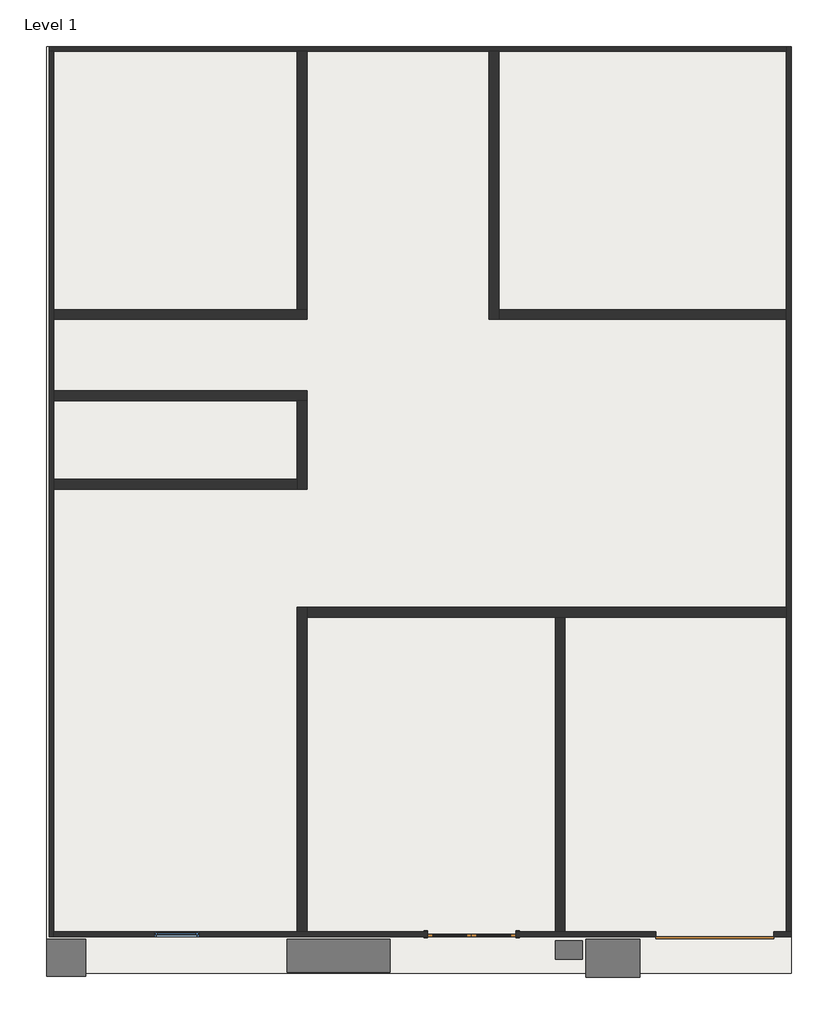
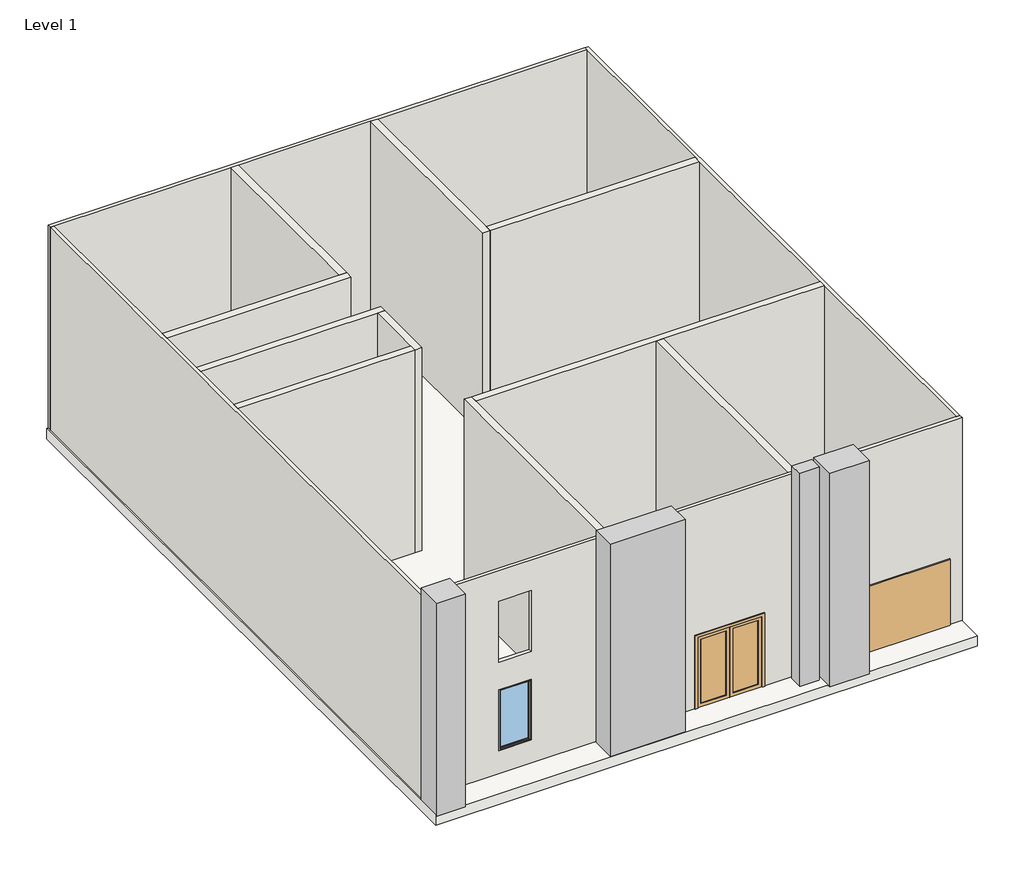
# One storey: 14 walls, 4 proxies, 2 doors, 1 slab, 1 window.
"""IFC4 building model written with IfcOpenShell, lengths in millimetres."""

from ifc_helpers import new_model, si_unit, frame, origin, origin_with_axes, place, context, project, spatial, polyline, outline, extrude, faceted_brep, transform, mapped, element, save
from components import generic_models_4_generic_models_4_105e3c89, generic_models_6_generic_models_6_789752cf, generic_models_7_generic_models_7_5b8c9dda, generic_models_8_generic_models_8_60fedc48, door_8f551b21, door_8b017a1a, window_8ce0b82f

model = new_model("IFC4")

# Units and contexts
model_context = context("Model", 3, world=origin())
ifc_project = project(units=[si_unit("LENGTHUNIT", "METRE", prefix="MILLI")], contexts=[model_context])

# Site, building, storey
site = spatial("IfcSite", under=ifc_project)
building = spatial("IfcBuilding", under=site)
storey = spatial("IfcBuildingStorey", under=building, Name="Level 1", Elevation=0.0)

# Proxies
placement = place(None, origin())
generic_models_4_generic_models_4_shape = generic_models_4_generic_models_4_105e3c89(model_context)
element("IfcBuildingElementProxy", 1, Name="Generic Models 4 : Generic Models 4", ObjectType="Generic Models 4 : Generic Models 4", at=placement, inside=storey, context=model_context, shape_type="MappedRepresentation", body=[
    mapped(generic_models_4_generic_models_4_shape, transform((0.0, 0.0, 0.0), x_axis=(1.0, 0.0, 0.0), y_axis=(0.0, 1.0, 0.0), z_axis=(0.0, 0.0, 1.0))),
])
generic_models_6_generic_models_6_shape = generic_models_6_generic_models_6_789752cf(model_context)
element("IfcBuildingElementProxy", 2, Name="Generic Models 6 : Generic Models 6", ObjectType="Generic Models 6 : Generic Models 6", at=placement, inside=storey, context=model_context, shape_type="MappedRepresentation", body=[
    mapped(generic_models_6_generic_models_6_shape, transform((0.0, 0.0, 0.0), x_axis=(1.0, 0.0, 0.0), y_axis=(0.0, 1.0, 0.0), z_axis=(0.0, 0.0, 1.0))),
])
generic_models_7_generic_models_7_shape = generic_models_7_generic_models_7_5b8c9dda(model_context)
element("IfcBuildingElementProxy", 3, Name="Generic Models 7 : Generic Models 7", ObjectType="Generic Models 7 : Generic Models 7", at=placement, inside=storey, context=model_context, shape_type="MappedRepresentation", body=[
    mapped(generic_models_7_generic_models_7_shape, transform((0.0, 0.0, 0.0), x_axis=(1.0, 0.0, 0.0), y_axis=(0.0, 1.0, 0.0), z_axis=(0.0, 0.0, 1.0))),
])
generic_models_8_generic_models_8_shape = generic_models_8_generic_models_8_60fedc48(model_context)
element("IfcBuildingElementProxy", 4, Name="Generic Models 8 : Generic Models 8", ObjectType="Generic Models 8 : Generic Models 8", at=placement, inside=storey, context=model_context, shape_type="MappedRepresentation", body=[
    mapped(generic_models_8_generic_models_8_shape, transform((0.0, 0.0, 0.0), x_axis=(1.0, 0.0, 0.0), y_axis=(0.0, 1.0, 0.0), z_axis=(0.0, 0.0, 1.0))),
])

# Doors
door_shape = door_8f551b21(model_context)
element("IfcDoor", 5, ObjectType="Door-Double-Glass : 72\" x 84\"", at=placement, inside=storey, context=model_context, shape_type="MappedRepresentation", body=[
    mapped(door_shape, transform((-1674.8069895, -8388.8167799, 0.0), x_axis=(-1.0, 0.0, 0.0), y_axis=(0.0, -1.0, 0.0), z_axis=(0.0, 0.0, 1.0))),
])
door_2_shape = door_8b017a1a(model_context)
element("IfcDoor", 6, ObjectType="Door-Overhead-Sectional : 8' x 6'-6\"", at=placement, inside=storey, context=model_context, shape_type="MappedRepresentation", body=[
    mapped(door_2_shape, transform((3354.3930105, -8391.1980299, 0.0), x_axis=(-1.0, 0.0, 0.0), y_axis=(0.0, -1.0, 0.0), z_axis=(0.0, 0.0, 1.0))),
])

# Slab
element("IfcSlab", 7, ObjectType="Generic - 12\"", at=placement, inside=storey, context=model_context, shape_type="SweptSolid", body=[
    extrude(outline(polyline([(4929.1930105, 9947.6019701), (4929.1930105, -9200.130387), (-10463.2069895, -9200.130387), (-10463.2069895, 9947.6019701), (4929.1930105, 9947.6019701)])), frame((0.0, 0.0, -304.8), z_axis=(0.0, 0.0, 1.0), x_axis=(1.0, 0.0, 0.0)), (0.0, 0.0, 1.0), 304.8),
])

# Walls
element("IfcWall", 8, ObjectType="Generic - 4\" Brick", at=placement, inside=storey, context=model_context, shape_type="Brep", body=[
    faceted_brep([(-10412.4069895, 9846.0019701, 0.0), (-10310.8069895, 9846.0019701, 0.0), (-5281.6069895, 9846.0019701, 0.0), (-5078.4069895, 9846.0019701, 0.0), (-1319.2069895, 9846.0019701, 0.0), (-1116.0069895, 9846.0019701, 0.0), (4827.5930105, 9846.0019701, 0.0), (4827.5930105, 9846.0019701, 6096.0), (-1116.0069895, 9846.0019701, 6096.0), (-1319.2069895, 9846.0019701, 6096.0), (-5078.4069895, 9846.0019701, 6096.0), (-5281.6069895, 9846.0019701, 6096.0), (-10310.8069895, 9846.0019701, 6096.0), (-10412.4069895, 9846.0019701, 6096.0), (-10412.4069895, 9947.6019701, 0.0), (-10412.4069895, 9947.6019701, 6096.0), (4827.5930105, 9947.6019701, 6096.0), (4827.5930105, 9947.6019701, 0.0)], [[[0, 1, 2, 3, 4, 5, 6, 7, 8, 9, 10, 11, 12, 13]], [[14, 15, 16, 17]], [[6, 5, 4, 3, 2, 1, 0, 14, 17]], [[0, 13, 15, 14]], [[7, 6, 17, 16]], [[13, 12, 11, 10, 9, 8, 7, 16, 15]]]),
])
element("IfcWall", 9, ObjectType="Generic - 4\" Brick", at=placement, inside=storey, context=model_context, shape_type="Brep", body=[
    faceted_brep([(-10310.8069895, -8441.9980299, 0.0), (-10310.8069895, -8340.3980299, 0.0), (-10310.8069895, 803.6019701, 0.0), (-10310.8069895, 1006.8019701, 0.0), (-10310.8069895, 2632.4019701, 0.0), (-10310.8069895, 2835.6019701, 0.0), (-10310.8069895, 4308.8019701, 0.0), (-10310.8069895, 4512.0019701, 0.0), (-10310.8069895, 9846.0019701, 0.0), (-10310.8069895, 9846.0019701, 6096.0), (-10310.8069895, 4512.0019701, 6096.0), (-10310.8069895, 4308.8019701, 6096.0), (-10310.8069895, 2835.6019701, 6096.0), (-10310.8069895, 2632.4019701, 6096.0), (-10310.8069895, 1006.8019701, 6096.0), (-10310.8069895, 803.6019701, 6096.0), (-10310.8069895, -8340.3980299, 6096.0), (-10310.8069895, -8441.9980299, 6096.0), (-10412.4069895, -8441.9980299, 0.0), (-10412.4069895, -8441.9980299, 6096.0), (-10412.4069895, 9846.0019701, 6096.0), (-10412.4069895, 9846.0019701, 0.0)], [[[0, 1, 2, 3, 4, 5, 6, 7, 8, 9, 10, 11, 12, 13, 14, 15, 16, 17]], [[18, 19, 20, 21]], [[8, 7, 6, 5, 4, 3, 2, 1, 0, 18, 21]], [[0, 17, 19, 18]], [[9, 8, 21, 20]], [[17, 16, 15, 14, 13, 12, 11, 10, 9, 20, 19]]]),
])
element("IfcWall", 10, ObjectType="Generic - 4\" Brick", at=placement, inside=storey, context=model_context, shape_type="Brep", body=[
    faceted_brep([(4929.1930105, -8340.3980299, 6096.0), (4929.1930105, -8340.3980299, 0.0), (4827.5930105, -8340.3980299, 0.0), (4573.5930105, -8340.3980299, 0.0), (4573.5930105, -8340.3980299, 1981.2), (2135.1930105, -8340.3980299, 1981.2), (2135.1930105, -8340.3980299, 0.0), (255.5930105, -8340.3980299, 0.0), (52.3930105, -8340.3980299, 0.0), (-760.4069895, -8340.3980299, 0.0), (-760.4069895, -8340.3980299, 2133.6), (-2589.2069895, -8340.3980299, 2133.6), (-2589.2069895, -8340.3980299, 0.0), (-5078.4069895, -8340.3980299, 0.0), (-5281.6069895, -8340.3980299, 0.0), (-10310.8069895, -8340.3980299, 0.0), (-10310.8069895, -8340.3980299, 6096.0), (-5281.6069895, -8340.3980299, 6096.0), (-5078.4069895, -8340.3980299, 6096.0), (52.3930105, -8340.3980299, 6096.0), (255.5930105, -8340.3980299, 6096.0), (4827.5930105, -8340.3980299, 6096.0), (-7313.6069895, -8340.3980299, 2518.9071751), (-8228.0069895, -8340.3980299, 2518.9071751), (-8228.0069895, -8340.3980299, 690.1071751), (-7313.6069895, -8340.3980299, 690.1071751), (-7313.6069895, -8340.3980299, 5181.6), (-8228.0069895, -8340.3980299, 5181.6), (-8228.0069895, -8340.3980299, 3352.8), (-7313.6069895, -8340.3980299, 3352.8), (4929.1930105, -8441.9980299, 0.0), (4929.1930105, -8441.9980299, 6096.0), (-10310.8069895, -8441.9980299, 6096.0), (-10310.8069895, -8441.9980299, 0.0), (-2589.2069895, -8441.9980299, 0.0), (-2589.2069895, -8441.9980299, 2133.6), (-760.4069895, -8441.9980299, 2133.6), (-760.4069895, -8441.9980299, 0.0), (2135.1930105, -8441.9980299, 0.0), (2135.1930105, -8441.9980299, 1981.2), (4573.5930105, -8441.9980299, 1981.2), (4573.5930105, -8441.9980299, 0.0), (-7313.6069895, -8441.9980299, 2518.9071751), (-7313.6069895, -8441.9980299, 690.1071751), (-8228.0069895, -8441.9980299, 690.1071751), (-8228.0069895, -8441.9980299, 2518.9071751), (-7313.6069895, -8441.9980299, 5181.6), (-7313.6069895, -8441.9980299, 3352.8), (-8228.0069895, -8441.9980299, 3352.8), (-8228.0069895, -8441.9980299, 5181.6)], [[[0, 1, 2, 3, 4, 5, 6, 7, 8, 9, 10, 11, 12, 13, 14, 15, 16, 17, 18, 19, 20, 21], [22, 23, 24, 25], [26, 27, 28, 29]], [[30, 31, 32, 33, 34, 35, 36, 37, 38, 39, 40, 41], [42, 43, 44, 45], [46, 47, 48, 49]], [[1, 30, 41, 3, 2]], [[33, 15, 14, 13, 12, 34]], [[37, 9, 8, 7, 6, 38]], [[1, 0, 31, 30]], [[16, 15, 33, 32]], [[0, 21, 20, 19, 18, 17, 16, 32, 31]], [[35, 34, 12, 11]], [[36, 35, 11, 10]], [[37, 36, 10, 9]], [[43, 42, 22, 25]], [[44, 43, 25, 24]], [[45, 44, 24, 23]], [[42, 45, 23, 22]], [[47, 46, 26, 29]], [[48, 47, 29, 28]], [[49, 48, 28, 27]], [[46, 49, 27, 26]], [[5, 39, 38, 6]], [[39, 5, 4, 40]], [[40, 4, 3, 41]]]),
])
element("IfcWall", 11, ObjectType="Generic - 4\" Brick", at=placement, inside=storey, context=model_context, shape_type="Brep", body=[
    faceted_brep([(4827.5930105, 9947.6019701, 0.0), (4827.5930105, 9846.0019701, 0.0), (4827.5930105, 4512.0019701, 0.0), (4827.5930105, 4308.8019701, 0.0), (4827.5930105, -1634.7980299, 0.0), (4827.5930105, -1837.9980299, 0.0), (4827.5930105, -8340.3980299, 0.0), (4827.5930105, -8340.3980299, 6096.0), (4827.5930105, -1837.9980299, 6096.0), (4827.5930105, -1634.7980299, 6096.0), (4827.5930105, 4308.8019701, 6096.0), (4827.5930105, 4512.0019701, 6096.0), (4827.5930105, 9846.0019701, 6096.0), (4827.5930105, 9947.6019701, 6096.0), (4929.1930105, 9947.6019701, 0.0), (4929.1930105, 9947.6019701, 6096.0), (4929.1930105, -8340.3980299, 6096.0), (4929.1930105, -8340.3980299, 0.0)], [[[0, 1, 2, 3, 4, 5, 6, 7, 8, 9, 10, 11, 12, 13]], [[14, 15, 16, 17]], [[6, 5, 4, 3, 2, 1, 0, 14, 17]], [[0, 13, 15, 14]], [[7, 6, 17, 16]], [[13, 12, 11, 10, 9, 8, 7, 16, 15]]]),
])
element("IfcWall", 12, ObjectType="Generic - 8\"", at=placement, inside=storey, context=model_context, shape_type="Brep", body=[
    faceted_brep([(-5078.4069895, -8340.3980299, 0.0), (-5078.4069895, -1837.9980299, 0.0), (-5078.4069895, -1634.7980299, 0.0), (-5078.4069895, -1634.7980299, 6096.0), (-5078.4069895, -1837.9980299, 6096.0), (-5078.4069895, -8340.3980299, 6096.0), (-5281.6069895, -8340.3980299, 0.0), (-5281.6069895, -8340.3980299, 6096.0), (-5281.6069895, -1634.7980299, 6096.0), (-5281.6069895, -1634.7980299, 0.0)], [[[0, 1, 2, 3, 4, 5]], [[6, 7, 8, 9]], [[2, 1, 0, 6, 9]], [[0, 5, 7, 6]], [[3, 2, 9, 8]], [[5, 4, 3, 8, 7]]]),
])
element("IfcWall", 13, ObjectType="Generic - 8\"", at=placement, inside=storey, context=model_context, shape_type="Brep", body=[
    faceted_brep([(-5078.4069895, -1837.9980299, 0.0), (52.3930105, -1837.9980299, 0.0), (255.5930105, -1837.9980299, 0.0), (4827.5930105, -1837.9980299, 0.0), (4827.5930105, -1837.9980299, 6096.0), (255.5930105, -1837.9980299, 6096.0), (52.3930105, -1837.9980299, 6096.0), (-5078.4069895, -1837.9980299, 6096.0), (-5078.4069895, -1634.7980299, 0.0), (-5078.4069895, -1634.7980299, 6096.0), (4827.5930105, -1634.7980299, 6096.0), (4827.5930105, -1634.7980299, 0.0)], [[[0, 1, 2, 3, 4, 5, 6, 7]], [[8, 9, 10, 11]], [[3, 2, 1, 0, 8, 11]], [[0, 7, 9, 8]], [[4, 3, 11, 10]], [[7, 6, 5, 4, 10, 9]]]),
])
element("IfcWall", 14, ObjectType="Generic - 8\"", at=placement, inside=storey, context=model_context, shape_type="SweptSolid", body=[
    extrude(outline(polyline([(52.3930105, -8340.3980299), (52.3930105, -1837.9980299), (255.5930105, -1837.9980299), (255.5930105, -8340.3980299), (52.3930105, -8340.3980299)])), origin_with_axes(), (0.0, 0.0, 1.0), 6096.0),
])
element("IfcWall", 15, ObjectType="Generic - 8\"", at=placement, inside=storey, context=model_context, shape_type="Brep", body=[
    faceted_brep([(-10310.8069895, 4308.8019701, 0.0), (-5078.4069895, 4308.8019701, 0.0), (-5078.4069895, 4308.8019701, 6096.0), (-10310.8069895, 4308.8019701, 6096.0), (-10310.8069895, 4512.0019701, 0.0), (-10310.8069895, 4512.0019701, 6096.0), (-5281.6069895, 4512.0019701, 6096.0), (-5078.4069895, 4512.0019701, 6096.0), (-5078.4069895, 4512.0019701, 0.0), (-5281.6069895, 4512.0019701, 0.0)], [[[0, 1, 2, 3]], [[4, 5, 6, 7, 8, 9]], [[1, 0, 4, 9, 8]], [[0, 3, 5, 4]], [[2, 1, 8, 7]], [[3, 2, 7, 6, 5]]]),
])
element("IfcWall", 16, ObjectType="Generic - 8\"", at=placement, inside=storey, context=model_context, shape_type="SweptSolid", body=[
    extrude(outline(polyline([(-5078.4069895, 9846.0019701), (-5078.4069895, 4512.0019701), (-5281.6069895, 4512.0019701), (-5281.6069895, 9846.0019701), (-5078.4069895, 9846.0019701)])), origin_with_axes(), (0.0, 0.0, 1.0), 6096.0),
])
element("IfcWall", 17, ObjectType="Generic - 8\"", at=placement, inside=storey, context=model_context, shape_type="Brep", body=[
    faceted_brep([(-10310.8069895, 2632.4019701, 0.0), (-5281.6069895, 2632.4019701, 0.0), (-5078.4069895, 2632.4019701, 0.0), (-5078.4069895, 2632.4019701, 6096.0), (-5281.6069895, 2632.4019701, 6096.0), (-10310.8069895, 2632.4019701, 6096.0), (-10310.8069895, 2835.6019701, 0.0), (-10310.8069895, 2835.6019701, 6096.0), (-5078.4069895, 2835.6019701, 6096.0), (-5078.4069895, 2835.6019701, 0.0)], [[[0, 1, 2, 3, 4, 5]], [[6, 7, 8, 9]], [[2, 1, 0, 6, 9]], [[0, 5, 7, 6]], [[3, 2, 9, 8]], [[5, 4, 3, 8, 7]]]),
])
element("IfcWall", 18, ObjectType="Generic - 8\"", at=placement, inside=storey, context=model_context, shape_type="Brep", body=[
    faceted_brep([(-5281.6069895, 2632.4019701, 0.0), (-5281.6069895, 1006.8019701, 0.0), (-5281.6069895, 803.6019701, 0.0), (-5281.6069895, 803.6019701, 6096.0), (-5281.6069895, 1006.8019701, 6096.0), (-5281.6069895, 2632.4019701, 6096.0), (-5078.4069895, 2632.4019701, 0.0), (-5078.4069895, 2632.4019701, 6096.0), (-5078.4069895, 803.6019701, 6096.0), (-5078.4069895, 803.6019701, 0.0)], [[[0, 1, 2, 3, 4, 5]], [[6, 7, 8, 9]], [[2, 1, 0, 6, 9]], [[0, 5, 7, 6]], [[3, 2, 9, 8]], [[5, 4, 3, 8, 7]]]),
])
element("IfcWall", 19, ObjectType="Generic - 8\"", at=placement, inside=storey, context=model_context, shape_type="SweptSolid", body=[
    extrude(outline(polyline([(-10310.8069895, 1006.8019701), (-5281.6069895, 1006.8019701), (-5281.6069895, 803.6019701), (-10310.8069895, 803.6019701), (-10310.8069895, 1006.8019701)])), origin_with_axes(), (0.0, 0.0, 1.0), 6096.0),
])
element("IfcWall", 20, ObjectType="Generic - 8\"", at=placement, inside=storey, context=model_context, shape_type="Brep", body=[
    faceted_brep([(-1319.2069895, 9846.0019701, 0.0), (-1319.2069895, 4308.8019701, 0.0), (-1319.2069895, 4308.8019701, 6096.0), (-1319.2069895, 9846.0019701, 6096.0), (-1116.0069895, 9846.0019701, 0.0), (-1116.0069895, 9846.0019701, 6096.0), (-1116.0069895, 4512.0019701, 6096.0), (-1116.0069895, 4308.8019701, 6096.0), (-1116.0069895, 4308.8019701, 0.0), (-1116.0069895, 4512.0019701, 0.0)], [[[0, 1, 2, 3]], [[4, 5, 6, 7, 8, 9]], [[1, 0, 4, 9, 8]], [[0, 3, 5, 4]], [[2, 1, 8, 7]], [[3, 2, 7, 6, 5]]]),
])
element("IfcWall", 21, ObjectType="Generic - 8\"", at=placement, inside=storey, context=model_context, shape_type="SweptSolid", body=[
    extrude(outline(polyline([(4827.5930105, 4308.8019701), (-1116.0069895, 4308.8019701), (-1116.0069895, 4512.0019701), (4827.5930105, 4512.0019701), (4827.5930105, 4308.8019701)])), origin_with_axes(), (0.0, 0.0, 1.0), 6096.0),
])

# Window
window_shape = window_8ce0b82f(model_context)
element("IfcWindow", 22, ObjectType="Fixed : 36\" x 72\"", at=placement, inside=storey, context=model_context, shape_type="MappedRepresentation", body=[
    mapped(window_shape, transform((-7732.7069895, -8391.1980299, 385.3071751), x_axis=(1.0, 0.0, 0.0), y_axis=(0.0, 1.0, 0.0), z_axis=(0.0, 0.0, 1.0))),
])

save(model, "model.ifc")

# Revit data of these elements
# Type "Door-Double-Glass : 72\" x 84\""
#   Type Mark = "8"
#   Construction Type Id = "opn-d45"
#   Assembly Code = "C1020"
#   Analytic Construction = "Wood frame, double glass door "
#   W = 3' - 0"
#   Thickness = 0' - 2"
#   Thermal Resistance (R) = 1.8150 (h·ft²·°F)/BTU
#   Swing Angle [instance default] = 90.00°
#   Heat Transfer Coefficient (U) = 0.5510 BTU/(h·ft²·°F)
#   Height = 7' - 0"
#   Bottom Rail = 0' - 4"
#   Top Rail = 0' - 4"
#   Stiles = 0' - 4"
#   Trim Projection = 0' - 1"
#   Trim Width = 0' - 3"
#   Width = 6' - 0"
#   Define Thermal Properties by = 1
#   Glazing = Glass
#   Panel Material = Wood - Birch - Solid Stained Light Low Gloss
#   Trim Material = Paint - Sienna
#   Visual Light Transmittance = 0
#   Solar Heat Gain Coefficient = 0
#   Function = (empty or 0)
#   Wall Closure = (empty or 0)
# Type "Door-Overhead-Sectional : 8' x 6'-6\""
#   Type Mark = "9"
#   Construction Type Id = "MDOOR"
#   Assembly Code = "B2030400"
#   Analytic Construction = "Metal"
#   Rough Width [instance default] = 8' - 0"
#   Rough Height [instance default] = 6' - 6"
#   Heat Transfer Coefficient (U) = 0.651978 BTU/(h·ft²·°F)
#   Height [instance default] = 6' - 6"
#   Thickness = 0' - 1 1/2"
#   Width [instance default] = 8' - 0"
#   Define Thermal Properties by = 1
#   Function = 1
#   Panel Material = Steel, Paint Finish, Ivory, Matte
#   Visual Light Transmittance = 0
#   Solar Heat Gain Coefficient = 0
#   Wall Closure = (empty or 0)
# Type "Generic - 12\""
#   Assembly Code = "B1010"
#   Function = 0
#   Layers, outside or top first: 1' - 0" no material (function 1)
# Type "Generic - 4\" Brick"
#   Assembly Code = "B2010"
#   Layers, outside or top first: 0' - 4" "Brick, Common" (function 1)
# Type "Generic - 8\""
#   Assembly Code = "B2010"
#   Layers, outside or top first: 0' - 8" no material (function 1)
# Type "Fixed : 36\" x 72\""
#   Type Mark = "9"
#   Construction Type Id = "GSP4R"
#   Assembly Code = "B2020100"
#   Analytic Construction = "1/8 in Pilkington single glazing"
#   Visual Light Transmittance = 0.9
#   Solar Heat Gain Coefficient = 0.78
#   Heat Transfer Coefficient (U) = 0.6496 BTU/(h·ft²·°F)
#   Height = 6' - 0"
#   Default Sill Height = 1' - 0"
#   Width = 3' - 0"
#   Window Inset = 0' - 0 3/4"
#   Define Thermal Properties by = 1
#   Glass Pane Material = Glass
#   Sash Material = Sash
#   Wall Closure = (empty or 0)
# Element 1 (IfcBuildingElementProxy, "Generic Models 4 : Generic Models 4")
#   Phase Created = New Construction
# Element 2 (IfcBuildingElementProxy, "Generic Models 6 : Generic Models 6")
#   Phase Created = New Construction
# Element 3 (IfcBuildingElementProxy, "Generic Models 7 : Generic Models 7")
#   Phase Created = New Construction
# Element 4 (IfcBuildingElementProxy, "Generic Models 8 : Generic Models 8")
#   Phase Created = New Construction
# Element 5 (IfcDoor, "Door-Double-Glass : 72\" x 84\"")
#   Swing Angle = 90.00°
#   Phase Created = New Construction
#   Materials on its faces: "Wood - Birch - Solid Stained Light Low Gloss", "Paint - Sienna", "Glass"
# Element 6 (IfcDoor, "Door-Overhead-Sectional : 8' x 6'-6\"")
#   Width = 8' - 0"
#   Rough Width = 8' - 0"
#   Rough Height = 6' - 6"
#   Height = 6' - 6"
#   Phase Created = New Construction
#   Materials on its faces: "Steel, Paint Finish, Ivory, Matte"
# Element 7 (IfcSlab, "Generic - 12\"")
#   Height Offset From Level = 0' - 0"
#   Phase Created = New Construction
#   Materials on its faces: "Default Floor"
# Elements 8, 9, 10, 11 (IfcWall, "Generic - 4\" Brick")
#   Top Offset = 0' - 0"
#   Base Offset = 0' - 0"
#   Unconnected Height = 20' - 0"
#   wall height = 20' - 0"
#   Phase Created = New Construction
#   Base Constraint = Level 1
#   Materials on its faces: "Brick, Common"
# Elements 12, 13, 14, 15, 16, 17, 18, 19, 20, 21 (IfcWall, "Generic - 8\"")
#   Top Offset = 0' - 0"
#   Base Offset = 0' - 0"
#   Unconnected Height = 20' - 0"
#   wall height = 20' - 0"
#   Phase Created = New Construction
#   Base Constraint = Level 1
#   Materials on its faces: "Default Wall"
# Element 22 (IfcWindow, "Fixed : 36\" x 72\"")
#   Mark = "1"
#   Phase Created = New Construction
#   Materials on its faces: "Sash", "Glass"
# Materials
#   "Glass": class "Glass", colour RGB 0 128 192, transparency 0.75, Description = "Soda Lime Glass", Cost = 0
#   "Wood - Birch - Solid Stained Light Low Gloss": class "Wood", colour RGB 210 159 95, transparency 0, Cost = 0
#   "Paint - Sienna": colour RGB 118 70 51, transparency 0, Cost = 0
#   "Steel, Paint Finish, Ivory, Matte": class "Metal", colour RGB 247 247 239, transparency 0, Description = "Steel, paint finish, ivory, matte", Cost = 0
#   "Brick, Common": class "Masonry", colour RGB 170 98 104, transparency 0, Description = "Common brick", Cost = 0
#   "Sash": class "Wood", colour RGB 224 178 126, transparency 0
#   "Default Floor": colour RGB 128 128 128, transparency 0
#   "Default Wall": colour RGB 128 128 128, transparency 0
